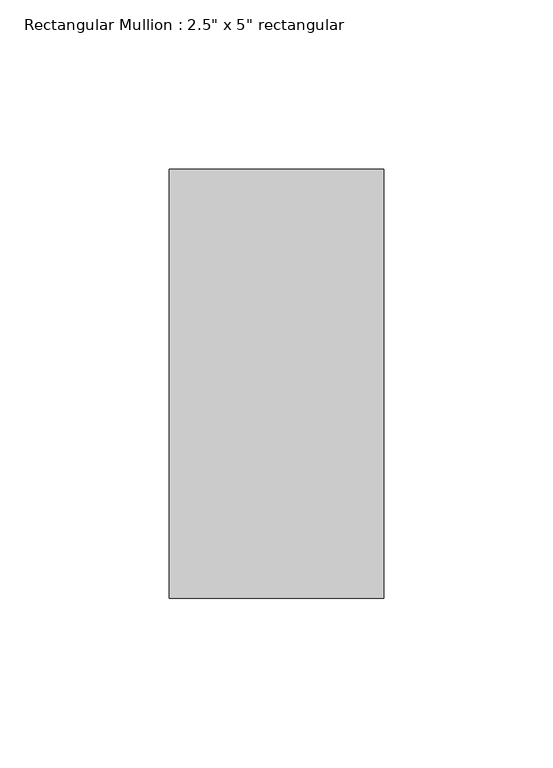
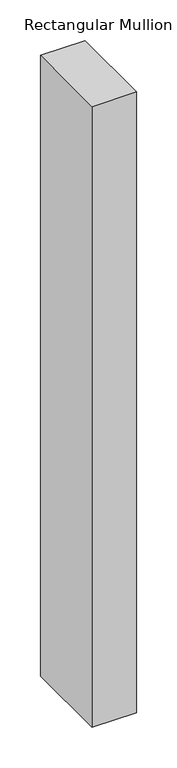
"""IFC4 building model written with IfcOpenShell, lengths in millimetres: member geometry."""

from ifc_helpers import new_model, si_unit, frame, origin, place, context, project, spatial, polyline, outline, extrude, source, transform, mapped, element, save


def member_c58de4df(model_context):
    return source(origin(), model_context, "Body", "SweptSolid", [
        extrude(outline(polyline([(31.75, 63.5), (31.75, -63.5), (-31.75, -63.5), (-31.75, 63.5), (31.75, 63.5)])), frame((0.0, 0.0, -934.0527116), z_axis=(0.0, 0.0, 1.0), x_axis=(1.0, 0.0, 0.0)), (0.0, 0.0, 1.0), 934.0527116),
    ])


if __name__ == "__main__":
    model = new_model("IFC4")
    model_context = context("Model", 3, world=origin())
    ifc_project = project(units=[si_unit("LENGTHUNIT", "METRE", prefix="MILLI")], contexts=[model_context])
    site = spatial("IfcSite", under=ifc_project)
    building = spatial("IfcBuilding", under=site)
    placement = place(None, origin())
    member_shape = member_c58de4df(model_context)
    element("IfcMember", 1, ObjectType="Rectangular Mullion : 2.5\" x 5\" rectangular", at=placement, inside=building, context=model_context, shape_type="MappedRepresentation", body=[
        mapped(member_shape, transform((0.0, 0.0, 0.0), x_axis=(1.0, 0.0, 0.0), y_axis=(0.0, 1.0, 0.0), z_axis=(0.0, 0.0, 1.0))),
    ])
    save(model, "model.ifc")

# Revit data of these elements
# Type "Rectangular Mullion : 2.5\" x 5\" rectangular"
#   built-in parameter 1007304 = 0.416667 (stored number, unit not read)
#   built-in parameter 1007301 = 0.104167 (stored number, unit not read)
#   built-in parameter 1007300 = 0.104167 (stored number, unit not read)
# Element 1 (IfcMember, "Rectangular Mullion : 2.5\" x 5\" rectangular")
#   Materials on its faces: "WINDOW FRAMING"
# Materials
#   "WINDOW FRAMING": class "Generic", colour RGB 120 120 120, transparency 0, Cost = 0
